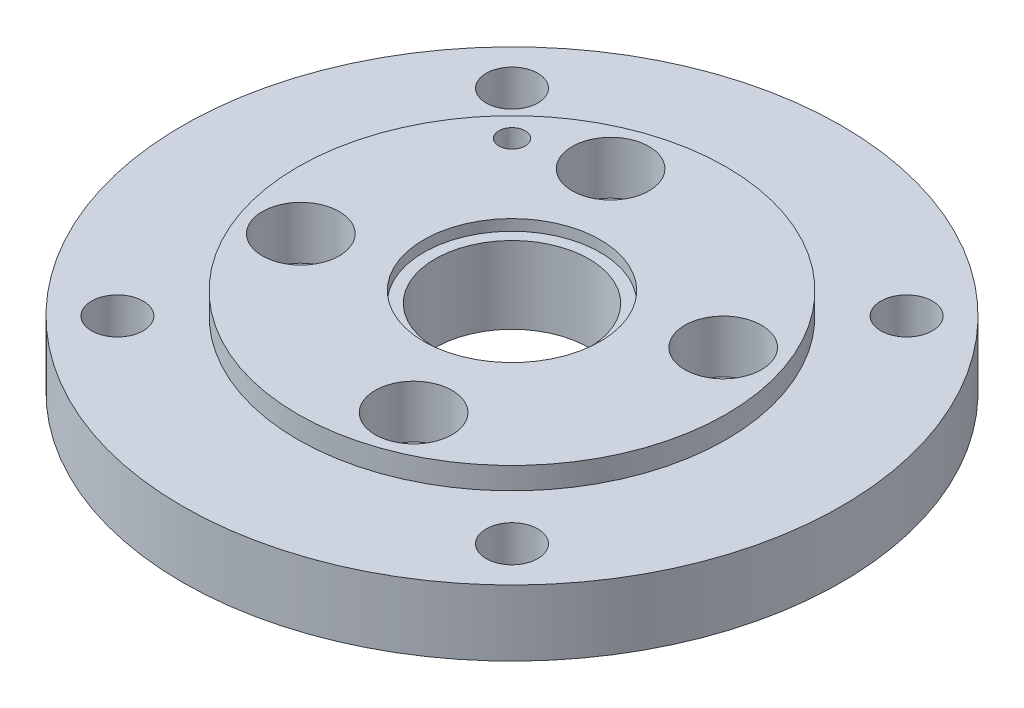
ISO-10303-21;
HEADER;
FILE_DESCRIPTION(('STEP AP214'),'2;1');
FILE_NAME('part.step','',(''),(''),'','','');
FILE_SCHEMA(('AUTOMOTIVE_DESIGN { 1 0 10303 214 1 1 1 1 }'));
ENDSEC;
DATA;
#1=APPLICATION_CONTEXT('core data for automotive mechanical design processes');
#2=APPLICATION_PROTOCOL_DEFINITION('international standard','automotive_design',2000,#1);
#3=PRODUCT_CONTEXT('',#1,'mechanical');
#4=PRODUCT('Part','Part','',(#3));
#5=PRODUCT_RELATED_PRODUCT_CATEGORY('part','',(#4));
#6=PRODUCT_DEFINITION_FORMATION('','',#4);
#7=PRODUCT_DEFINITION_CONTEXT('part definition',#1,'design');
#8=PRODUCT_DEFINITION('design','',#6,#7);
#9=PRODUCT_DEFINITION_SHAPE('','',#8);
#10=(LENGTH_UNIT() NAMED_UNIT(*) SI_UNIT(.MILLI.,.METRE.));
#11=(NAMED_UNIT(*) PLANE_ANGLE_UNIT() SI_UNIT($,.RADIAN.));
#12=(NAMED_UNIT(*) SI_UNIT($,.STERADIAN.) SOLID_ANGLE_UNIT());
#13=UNCERTAINTY_MEASURE_WITH_UNIT(LENGTH_MEASURE(1.E-05),#10,'distance_accuracy_value','');
#14=(GEOMETRIC_REPRESENTATION_CONTEXT(3) GLOBAL_UNCERTAINTY_ASSIGNED_CONTEXT((#13)) GLOBAL_UNIT_ASSIGNED_CONTEXT((#10,
#11,#12)) REPRESENTATION_CONTEXT('',''));
#15=CARTESIAN_POINT('',(0.,0.,0.));
#16=DIRECTION('',(0.,0.,1.));
#17=DIRECTION('',(1.,0.,0.));
#18=AXIS2_PLACEMENT_3D('',#15,#16,#17);
#19=CARTESIAN_POINT('',(0.,0.,0.));
#20=DIRECTION('',(0.,1.,0.));
#21=DIRECTION('',(0.,0.,1.));
#22=AXIS2_PLACEMENT_3D('',#19,#20,#21);
#23=PLANE('',#22);
#24=CARTESIAN_POINT('',(-60.,0.,-60.));
#25=DIRECTION('',(0.,1.,0.));
#26=DIRECTION('',(0.,0.,1.));
#27=AXIS2_PLACEMENT_3D('',#24,#25,#26);
#28=CIRCLE('',#27,6.);
#29=CARTESIAN_POINT('',(-60.,0.,-54.));
#30=VERTEX_POINT('',#29);
#31=EDGE_CURVE('E417',#30,#30,#28,.T.);
#32=ORIENTED_EDGE('',*,*,#31,.F.);
#33=EDGE_LOOP('',(#32));
#34=FACE_BOUND('',#33,.T.);
#35=CARTESIAN_POINT('',(-70.476946558943,0.,25.6515107494257));
#36=DIRECTION('',(0.,1.,0.));
#37=DIRECTION('',(0.,0.,1.));
#38=AXIS2_PLACEMENT_3D('',#35,#36,#37);
#39=CIRCLE('',#38,17.5);
#40=CARTESIAN_POINT('',(-70.476946558943,0.,43.1515107494257));
#41=VERTEX_POINT('',#40);
#42=EDGE_CURVE('E74',#41,#41,#39,.F.);
#43=ORIENTED_EDGE('',*,*,#42,.T.);
#44=EDGE_LOOP('',(#43));
#45=FACE_BOUND('',#44,.T.);
#46=CARTESIAN_POINT('',(25.686255304837,0.,70.4642908742771));
#47=DIRECTION('',(0.,1.,0.));
#48=DIRECTION('',(0.,0.,1.));
#49=AXIS2_PLACEMENT_3D('',#46,#47,#48);
#50=CIRCLE('',#49,17.5);
#51=CARTESIAN_POINT('',(25.686255304837,0.,87.9642908742771));
#52=VERTEX_POINT('',#51);
#53=EDGE_CURVE('E64',#52,#52,#50,.F.);
#54=ORIENTED_EDGE('',*,*,#53,.T.);
#55=EDGE_LOOP('',(#54));
#56=FACE_BOUND('',#55,.T.);
#57=CARTESIAN_POINT('',(0.,0.,0.));
#58=DIRECTION('',(0.,1.,0.));
#59=DIRECTION('',(0.,0.,1.));
#60=AXIS2_PLACEMENT_3D('',#57,#58,#59);
#61=CIRCLE('',#60,40.15);
#62=CARTESIAN_POINT('',(0.,0.,40.15));
#63=VERTEX_POINT('',#62);
#64=EDGE_CURVE('E113',#63,#63,#61,.T.);
#65=ORIENTED_EDGE('',*,*,#64,.F.);
#66=EDGE_LOOP('',(#65));
#67=FACE_BOUND('',#66,.T.);
#68=CARTESIAN_POINT('',(0.,0.,0.));
#69=DIRECTION('',(0.,1.,0.));
#70=DIRECTION('',(0.,0.,1.));
#71=AXIS2_PLACEMENT_3D('',#68,#69,#70);
#72=CIRCLE('',#71,97.5);
#73=CARTESIAN_POINT('',(0.,0.,97.5));
#74=VERTEX_POINT('',#73);
#75=EDGE_CURVE('E101',#74,#74,#72,.T.);
#76=ORIENTED_EDGE('',*,*,#75,.T.);
#77=EDGE_LOOP('',(#76));
#78=FACE_BOUND('',#77,.T.);
#79=CARTESIAN_POINT('',(70.4769465589431,0.,-25.6515107494252));
#80=DIRECTION('',(0.,1.,0.));
#81=DIRECTION('',(0.,0.,1.));
#82=AXIS2_PLACEMENT_3D('',#79,#80,#81);
#83=CIRCLE('',#82,17.5);
#84=CARTESIAN_POINT('',(70.4769465589431,0.,-8.15151074942521));
#85=VERTEX_POINT('',#84);
#86=EDGE_CURVE('E128',#85,#85,#83,.T.);
#87=ORIENTED_EDGE('',*,*,#86,.F.);
#88=EDGE_LOOP('',(#87));
#89=FACE_BOUND('',#88,.T.);
#90=CARTESIAN_POINT('',(-25.616759958528,0.,-70.4895851117536));
#91=DIRECTION('',(0.,1.,0.));
#92=DIRECTION('',(0.,0.,1.));
#93=AXIS2_PLACEMENT_3D('',#90,#91,#92);
#94=CIRCLE('',#93,17.5);
#95=CARTESIAN_POINT('',(-25.616759958528,0.,-52.9895851117536));
#96=VERTEX_POINT('',#95);
#97=EDGE_CURVE('E131',#96,#96,#94,.T.);
#98=ORIENTED_EDGE('',*,*,#97,.F.);
#99=EDGE_LOOP('',(#98));
#100=FACE_BOUND('',#99,.T.);
#101=ADVANCED_FACE('F40',(#34,#45,#56,#67,#78,#89,#100),#23,.T.);
#102=CARTESIAN_POINT('',(0.,-40.,0.));
#103=DIRECTION('',(0.,1.,0.));
#104=DIRECTION('',(0.,0.,1.));
#105=AXIS2_PLACEMENT_3D('',#102,#103,#104);
#106=CYLINDRICAL_SURFACE('',#105,150.);
#107=CARTESIAN_POINT('',(0.,-40.,0.));
#108=DIRECTION('',(0.,1.,0.));
#109=DIRECTION('',(0.,0.,1.));
#110=AXIS2_PLACEMENT_3D('',#107,#108,#109);
#111=CIRCLE('',#110,150.);
#112=CARTESIAN_POINT('',(0.,-40.,150.));
#113=VERTEX_POINT('',#112);
#114=EDGE_CURVE('E10',#113,#113,#111,.T.);
#115=ORIENTED_EDGE('',*,*,#114,.T.);
#116=EDGE_LOOP('',(#115));
#117=FACE_BOUND('',#116,.T.);
#118=CARTESIAN_POINT('',(0.,-10.,0.));
#119=DIRECTION('',(0.,1.,0.));
#120=DIRECTION('',(0.,0.,1.));
#121=AXIS2_PLACEMENT_3D('',#118,#119,#120);
#122=CIRCLE('',#121,150.);
#123=CARTESIAN_POINT('',(0.,-10.,150.));
#124=VERTEX_POINT('',#123);
#125=EDGE_CURVE('E110',#124,#124,#122,.T.);
#126=ORIENTED_EDGE('',*,*,#125,.F.);
#127=EDGE_LOOP('',(#126));
#128=FACE_BOUND('',#127,.T.);
#129=ADVANCED_FACE('F39',(#117,#128),#106,.T.);
#130=CARTESIAN_POINT('',(0.,-40.,0.));
#131=DIRECTION('',(0.,1.,0.));
#132=DIRECTION('',(0.,0.,1.));
#133=AXIS2_PLACEMENT_3D('',#130,#131,#132);
#134=CYLINDRICAL_SURFACE('',#133,35.);
#135=CARTESIAN_POINT('',(0.,-40.,0.));
#136=DIRECTION('',(0.,1.,0.));
#137=DIRECTION('',(0.,0.,1.));
#138=AXIS2_PLACEMENT_3D('',#135,#136,#137);
#139=CIRCLE('',#138,35.);
#140=CARTESIAN_POINT('',(0.,-40.,35.));
#141=VERTEX_POINT('',#140);
#142=EDGE_CURVE('E44',#141,#141,#139,.T.);
#143=ORIENTED_EDGE('',*,*,#142,.F.);
#144=EDGE_LOOP('',(#143));
#145=FACE_BOUND('',#144,.T.);
#146=CARTESIAN_POINT('',(0.,-5.,0.));
#147=DIRECTION('',(0.,1.,0.));
#148=DIRECTION('',(0.,0.,1.));
#149=AXIS2_PLACEMENT_3D('',#146,#147,#148);
#150=CIRCLE('',#149,35.);
#151=CARTESIAN_POINT('',(0.,-5.,35.));
#152=VERTEX_POINT('',#151);
#153=EDGE_CURVE('E115',#152,#152,#150,.T.);
#154=ORIENTED_EDGE('',*,*,#153,.T.);
#155=EDGE_LOOP('',(#154));
#156=FACE_BOUND('',#155,.T.);
#157=ADVANCED_FACE('F204',(#145,#156),#134,.F.);
#158=CARTESIAN_POINT('',(0.,-40.,0.));
#159=DIRECTION('',(0.,1.,0.));
#160=DIRECTION('',(0.,0.,1.));
#161=AXIS2_PLACEMENT_3D('',#158,#159,#160);
#162=PLANE('',#161);
#163=CARTESIAN_POINT('',(-60.,-40.,-60.));
#164=DIRECTION('',(0.,1.,0.));
#165=DIRECTION('',(0.,0.,1.));
#166=AXIS2_PLACEMENT_3D('',#163,#164,#165);
#167=CIRCLE('',#166,6.);
#168=CARTESIAN_POINT('',(-60.,-40.,-54.));
#169=VERTEX_POINT('',#168);
#170=EDGE_CURVE('E216',#169,#169,#167,.T.);
#171=ORIENTED_EDGE('',*,*,#170,.T.);
#172=EDGE_LOOP('',(#171));
#173=FACE_BOUND('',#172,.T.);
#174=CARTESIAN_POINT('',(70.4769465589431,-40.,-25.6515107494252));
#175=DIRECTION('',(0.,1.,0.));
#176=DIRECTION('',(0.,0.,1.));
#177=AXIS2_PLACEMENT_3D('',#174,#175,#176);
#178=CIRCLE('',#177,11.5);
#179=CARTESIAN_POINT('',(70.4769465589431,-40.,-14.1515107494252));
#180=VERTEX_POINT('',#179);
#181=EDGE_CURVE('E59',#180,#180,#178,.T.);
#182=ORIENTED_EDGE('',*,*,#181,.T.);
#183=EDGE_LOOP('',(#182));
#184=FACE_BOUND('',#183,.T.);
#185=CARTESIAN_POINT('',(-70.4074512126341,-40.,25.6262165119488));
#186=DIRECTION('',(0.,1.,0.));
#187=DIRECTION('',(0.,0.,-1.));
#188=AXIS2_PLACEMENT_3D('',#185,#186,#187);
#189=CIRCLE('',#188,11.5);
#190=CARTESIAN_POINT('',(-70.4074512126341,-40.,14.1262165119488));
#191=VERTEX_POINT('',#190);
#192=EDGE_CURVE('E224',#191,#191,#189,.T.);
#193=ORIENTED_EDGE('',*,*,#192,.T.);
#194=EDGE_LOOP('',(#193));
#195=FACE_BOUND('',#194,.T.);
#196=CARTESIAN_POINT('',(-25.616759958528,-40.,-70.4895851117536));
#197=DIRECTION('',(0.,1.,0.));
#198=DIRECTION('',(0.,0.,1.));
#199=AXIS2_PLACEMENT_3D('',#196,#197,#198);
#200=CIRCLE('',#199,11.5);
#201=CARTESIAN_POINT('',(-25.616759958528,-40.,-58.9895851117536));
#202=VERTEX_POINT('',#201);
#203=EDGE_CURVE('E230',#202,#202,#200,.T.);
#204=ORIENTED_EDGE('',*,*,#203,.T.);
#205=EDGE_LOOP('',(#204));
#206=FACE_BOUND('',#205,.T.);
#207=CARTESIAN_POINT('',(25.686255304837,-40.,70.4642908742771));
#208=DIRECTION('',(0.,1.,0.));
#209=DIRECTION('',(0.,0.,-1.));
#210=AXIS2_PLACEMENT_3D('',#207,#208,#209);
#211=CIRCLE('',#210,11.5000000000005);
#212=CARTESIAN_POINT('',(25.686255304837,-40.,58.9642908742766));
#213=VERTEX_POINT('',#212);
#214=EDGE_CURVE('E231',#213,#213,#211,.T.);
#215=ORIENTED_EDGE('',*,*,#214,.T.);
#216=EDGE_LOOP('',(#215));
#217=FACE_BOUND('',#216,.T.);
#218=CARTESIAN_POINT('',(89.8025612106914,-40.,89.8025612106917));
#219=DIRECTION('',(0.,1.,0.));
#220=DIRECTION('',(0.,0.,-1.));
#221=AXIS2_PLACEMENT_3D('',#218,#219,#220);
#222=CIRCLE('',#221,11.75);
#223=CARTESIAN_POINT('',(89.8025612106914,-40.,78.0525612106917));
#224=VERTEX_POINT('',#223);
#225=EDGE_CURVE('E93',#224,#224,#222,.T.);
#226=ORIENTED_EDGE('',*,*,#225,.T.);
#227=EDGE_LOOP('',(#226));
#228=FACE_BOUND('',#227,.T.);
#229=CARTESIAN_POINT('',(-89.8025612106914,-40.,89.8025612106917));
#230=DIRECTION('',(0.,1.,0.));
#231=DIRECTION('',(0.,0.,1.));
#232=AXIS2_PLACEMENT_3D('',#229,#230,#231);
#233=CIRCLE('',#232,11.75);
#234=CARTESIAN_POINT('',(-89.8025612106914,-40.,101.552561210692));
#235=VERTEX_POINT('',#234);
#236=EDGE_CURVE('E85',#235,#235,#233,.T.);
#237=ORIENTED_EDGE('',*,*,#236,.T.);
#238=EDGE_LOOP('',(#237));
#239=FACE_BOUND('',#238,.T.);
#240=CARTESIAN_POINT('',(-89.8025612106914,-40.,-89.8025612106917));
#241=DIRECTION('',(0.,1.,0.));
#242=DIRECTION('',(0.,0.,-1.));
#243=AXIS2_PLACEMENT_3D('',#240,#241,#242);
#244=CIRCLE('',#243,11.75);
#245=CARTESIAN_POINT('',(-89.8025612106914,-40.,-101.552561210692));
#246=VERTEX_POINT('',#245);
#247=EDGE_CURVE('E76',#246,#246,#244,.T.);
#248=ORIENTED_EDGE('',*,*,#247,.T.);
#249=EDGE_LOOP('',(#248));
#250=FACE_BOUND('',#249,.T.);
#251=CARTESIAN_POINT('',(89.8025612106914,-40.,-89.8025612106917));
#252=DIRECTION('',(0.,1.,0.));
#253=DIRECTION('',(0.,0.,1.));
#254=AXIS2_PLACEMENT_3D('',#251,#252,#253);
#255=CIRCLE('',#254,11.75);
#256=CARTESIAN_POINT('',(89.8025612106914,-40.,-78.0525612106917));
#257=VERTEX_POINT('',#256);
#258=EDGE_CURVE('E98',#257,#257,#255,.T.);
#259=ORIENTED_EDGE('',*,*,#258,.T.);
#260=EDGE_LOOP('',(#259));
#261=FACE_BOUND('',#260,.T.);
#262=ORIENTED_EDGE('',*,*,#142,.T.);
#263=EDGE_LOOP('',(#262));
#264=FACE_BOUND('',#263,.T.);
#265=ORIENTED_EDGE('',*,*,#114,.F.);
#266=EDGE_LOOP('',(#265));
#267=FACE_BOUND('',#266,.T.);
#268=ADVANCED_FACE('F205',(#173,#184,#195,#206,#217,#228,#239,#250,#261,#264,#267),#162,.F.);
#269=CARTESIAN_POINT('',(0.,-5.,0.));
#270=DIRECTION('',(0.,1.,0.));
#271=DIRECTION('',(0.,0.,1.));
#272=AXIS2_PLACEMENT_3D('',#269,#270,#271);
#273=CYLINDRICAL_SURFACE('',#272,40.15);
#274=CARTESIAN_POINT('',(0.,-5.,0.));
#275=DIRECTION('',(0.,1.,0.));
#276=DIRECTION('',(0.,0.,1.));
#277=AXIS2_PLACEMENT_3D('',#274,#275,#276);
#278=CIRCLE('',#277,40.15);
#279=CARTESIAN_POINT('',(0.,-5.,40.15));
#280=VERTEX_POINT('',#279);
#281=EDGE_CURVE('E49',#280,#280,#278,.T.);
#282=ORIENTED_EDGE('',*,*,#281,.F.);
#283=EDGE_LOOP('',(#282));
#284=FACE_BOUND('',#283,.T.);
#285=ORIENTED_EDGE('',*,*,#64,.T.);
#286=EDGE_LOOP('',(#285));
#287=FACE_BOUND('',#286,.T.);
#288=ADVANCED_FACE('F119',(#284,#287),#273,.F.);
#289=CARTESIAN_POINT('',(0.,-5.,0.));
#290=DIRECTION('',(0.,1.,0.));
#291=DIRECTION('',(0.,0.,1.));
#292=AXIS2_PLACEMENT_3D('',#289,#290,#291);
#293=PLANE('',#292);
#294=ORIENTED_EDGE('',*,*,#153,.F.);
#295=EDGE_LOOP('',(#294));
#296=FACE_BOUND('',#295,.T.);
#297=ORIENTED_EDGE('',*,*,#281,.T.);
#298=EDGE_LOOP('',(#297));
#299=FACE_BOUND('',#298,.T.);
#300=ADVANCED_FACE('F195',(#296,#299),#293,.T.);
#301=CARTESIAN_POINT('',(0.,-10.,0.));
#302=DIRECTION('',(0.,1.,0.));
#303=DIRECTION('',(0.,0.,1.));
#304=AXIS2_PLACEMENT_3D('',#301,#302,#303);
#305=PLANE('',#304);
#306=CARTESIAN_POINT('',(89.8025612106914,-10.,89.8025612106917));
#307=DIRECTION('',(0.,1.,0.));
#308=DIRECTION('',(0.,0.,-1.));
#309=AXIS2_PLACEMENT_3D('',#306,#307,#308);
#310=CIRCLE('',#309,11.75);
#311=CARTESIAN_POINT('',(89.8025612106914,-10.,78.0525612106917));
#312=VERTEX_POINT('',#311);
#313=EDGE_CURVE('E94',#312,#312,#310,.T.);
#314=ORIENTED_EDGE('',*,*,#313,.F.);
#315=EDGE_LOOP('',(#314));
#316=FACE_BOUND('',#315,.T.);
#317=CARTESIAN_POINT('',(-89.8025612106914,-10.,89.8025612106917));
#318=DIRECTION('',(0.,1.,0.));
#319=DIRECTION('',(0.,0.,1.));
#320=AXIS2_PLACEMENT_3D('',#317,#318,#319);
#321=CIRCLE('',#320,11.75);
#322=CARTESIAN_POINT('',(-89.8025612106914,-10.,101.552561210692));
#323=VERTEX_POINT('',#322);
#324=EDGE_CURVE('E86',#323,#323,#321,.T.);
#325=ORIENTED_EDGE('',*,*,#324,.F.);
#326=EDGE_LOOP('',(#325));
#327=FACE_BOUND('',#326,.T.);
#328=CARTESIAN_POINT('',(-89.8025612106914,-10.,-89.8025612106917));
#329=DIRECTION('',(0.,1.,0.));
#330=DIRECTION('',(0.,0.,-1.));
#331=AXIS2_PLACEMENT_3D('',#328,#329,#330);
#332=CIRCLE('',#331,11.75);
#333=CARTESIAN_POINT('',(-89.8025612106914,-10.,-101.552561210692));
#334=VERTEX_POINT('',#333);
#335=EDGE_CURVE('E82',#334,#334,#332,.T.);
#336=ORIENTED_EDGE('',*,*,#335,.F.);
#337=EDGE_LOOP('',(#336));
#338=FACE_BOUND('',#337,.T.);
#339=CARTESIAN_POINT('',(89.8025612106914,-10.,-89.8025612106917));
#340=DIRECTION('',(0.,1.,0.));
#341=DIRECTION('',(0.,0.,1.));
#342=AXIS2_PLACEMENT_3D('',#339,#340,#341);
#343=CIRCLE('',#342,11.75);
#344=CARTESIAN_POINT('',(89.8025612106914,-10.,-78.0525612106917));
#345=VERTEX_POINT('',#344);
#346=EDGE_CURVE('E81',#345,#345,#343,.T.);
#347=ORIENTED_EDGE('',*,*,#346,.F.);
#348=EDGE_LOOP('',(#347));
#349=FACE_BOUND('',#348,.T.);
#350=CARTESIAN_POINT('',(0.,-10.,0.));
#351=DIRECTION('',(0.,1.,0.));
#352=DIRECTION('',(0.,0.,1.));
#353=AXIS2_PLACEMENT_3D('',#350,#351,#352);
#354=CIRCLE('',#353,97.5);
#355=CARTESIAN_POINT('',(0.,-10.,97.5));
#356=VERTEX_POINT('',#355);
#357=EDGE_CURVE('E102',#356,#356,#354,.T.);
#358=ORIENTED_EDGE('',*,*,#357,.F.);
#359=EDGE_LOOP('',(#358));
#360=FACE_BOUND('',#359,.T.);
#361=ORIENTED_EDGE('',*,*,#125,.T.);
#362=EDGE_LOOP('',(#361));
#363=FACE_BOUND('',#362,.T.);
#364=ADVANCED_FACE('F191',(#316,#327,#338,#349,#360,#363),#305,.T.);
#365=CARTESIAN_POINT('',(0.,-10.,0.));
#366=DIRECTION('',(0.,1.,0.));
#367=DIRECTION('',(0.,0.,1.));
#368=AXIS2_PLACEMENT_3D('',#365,#366,#367);
#369=CYLINDRICAL_SURFACE('',#368,97.5);
#370=ORIENTED_EDGE('',*,*,#357,.T.);
#371=EDGE_LOOP('',(#370));
#372=FACE_BOUND('',#371,.T.);
#373=ORIENTED_EDGE('',*,*,#75,.F.);
#374=EDGE_LOOP('',(#373));
#375=FACE_BOUND('',#374,.T.);
#376=ADVANCED_FACE('F190',(#372,#375),#369,.T.);
#377=CARTESIAN_POINT('',(89.8025612106914,-40.,-89.8025612106917));
#378=DIRECTION('',(0.,1.,0.));
#379=DIRECTION('',(0.,0.,1.));
#380=AXIS2_PLACEMENT_3D('',#377,#378,#379);
#381=CYLINDRICAL_SURFACE('',#380,11.75);
#382=ORIENTED_EDGE('',*,*,#258,.F.);
#383=EDGE_LOOP('',(#382));
#384=FACE_BOUND('',#383,.T.);
#385=ORIENTED_EDGE('',*,*,#346,.T.);
#386=EDGE_LOOP('',(#385));
#387=FACE_BOUND('',#386,.T.);
#388=ADVANCED_FACE('F177',(#384,#387),#381,.F.);
#389=CARTESIAN_POINT('',(-89.8025612106914,-40.,-89.8025612106917));
#390=DIRECTION('',(0.,1.,0.));
#391=DIRECTION('',(0.,0.,1.));
#392=AXIS2_PLACEMENT_3D('',#389,#390,#391);
#393=CYLINDRICAL_SURFACE('',#392,11.75);
#394=ORIENTED_EDGE('',*,*,#247,.F.);
#395=EDGE_LOOP('',(#394));
#396=FACE_BOUND('',#395,.T.);
#397=ORIENTED_EDGE('',*,*,#335,.T.);
#398=EDGE_LOOP('',(#397));
#399=FACE_BOUND('',#398,.T.);
#400=ADVANCED_FACE('F171',(#396,#399),#393,.F.);
#401=CARTESIAN_POINT('',(-89.8025612106914,-40.,89.8025612106917));
#402=DIRECTION('',(0.,1.,0.));
#403=DIRECTION('',(0.,0.,1.));
#404=AXIS2_PLACEMENT_3D('',#401,#402,#403);
#405=CYLINDRICAL_SURFACE('',#404,11.75);
#406=ORIENTED_EDGE('',*,*,#236,.F.);
#407=EDGE_LOOP('',(#406));
#408=FACE_BOUND('',#407,.T.);
#409=ORIENTED_EDGE('',*,*,#324,.T.);
#410=EDGE_LOOP('',(#409));
#411=FACE_BOUND('',#410,.T.);
#412=ADVANCED_FACE('F176',(#408,#411),#405,.F.);
#413=CARTESIAN_POINT('',(89.8025612106914,-40.,89.8025612106917));
#414=DIRECTION('',(0.,1.,0.));
#415=DIRECTION('',(0.,0.,1.));
#416=AXIS2_PLACEMENT_3D('',#413,#414,#415);
#417=CYLINDRICAL_SURFACE('',#416,11.75);
#418=ORIENTED_EDGE('',*,*,#225,.F.);
#419=EDGE_LOOP('',(#418));
#420=FACE_BOUND('',#419,.T.);
#421=ORIENTED_EDGE('',*,*,#313,.T.);
#422=EDGE_LOOP('',(#421));
#423=FACE_BOUND('',#422,.T.);
#424=ADVANCED_FACE('F173',(#420,#423),#417,.F.);
#425=CARTESIAN_POINT('',(25.686255304837,-24.,70.4642908742771));
#426=DIRECTION('',(0.,1.,0.));
#427=DIRECTION('',(0.,0.,1.));
#428=AXIS2_PLACEMENT_3D('',#425,#426,#427);
#429=CYLINDRICAL_SURFACE('',#428,17.5);
#430=CARTESIAN_POINT('',(25.686255304837,-24.,70.4642908742771));
#431=DIRECTION('',(0.,1.,0.));
#432=DIRECTION('',(0.,0.,1.));
#433=AXIS2_PLACEMENT_3D('',#430,#431,#432);
#434=CIRCLE('',#433,17.5);
#435=CARTESIAN_POINT('',(25.686255304837,-24.,87.9642908742771));
#436=VERTEX_POINT('',#435);
#437=EDGE_CURVE('E68',#436,#436,#434,.F.);
#438=ORIENTED_EDGE('',*,*,#437,.T.);
#439=EDGE_LOOP('',(#438));
#440=FACE_BOUND('',#439,.T.);
#441=ORIENTED_EDGE('',*,*,#53,.F.);
#442=EDGE_LOOP('',(#441));
#443=FACE_BOUND('',#442,.T.);
#444=ADVANCED_FACE('F164',(#440,#443),#429,.F.);
#445=CARTESIAN_POINT('',(0.,-24.,0.));
#446=DIRECTION('',(0.,1.,0.));
#447=DIRECTION('',(0.,0.,1.));
#448=AXIS2_PLACEMENT_3D('',#445,#446,#447);
#449=PLANE('',#448);
#450=CARTESIAN_POINT('',(25.686255304837,-24.,70.4642908742771));
#451=DIRECTION('',(0.,1.,0.));
#452=DIRECTION('',(0.,0.,1.));
#453=AXIS2_PLACEMENT_3D('',#450,#451,#452);
#454=CIRCLE('',#453,11.5000000000005);
#455=CARTESIAN_POINT('',(25.686255304837,-24.,81.9642908742776));
#456=VERTEX_POINT('',#455);
#457=EDGE_CURVE('E41',#456,#456,#454,.T.);
#458=ORIENTED_EDGE('',*,*,#457,.F.);
#459=EDGE_LOOP('',(#458));
#460=FACE_BOUND('',#459,.T.);
#461=ORIENTED_EDGE('',*,*,#437,.F.);
#462=EDGE_LOOP('',(#461));
#463=FACE_BOUND('',#462,.T.);
#464=ADVANCED_FACE('F153',(#460,#463),#449,.T.);
#465=CARTESIAN_POINT('',(-70.476946558943,-24.,25.6515107494257));
#466=DIRECTION('',(0.,1.,0.));
#467=DIRECTION('',(0.,0.,1.));
#468=AXIS2_PLACEMENT_3D('',#465,#466,#467);
#469=CYLINDRICAL_SURFACE('',#468,17.5);
#470=CARTESIAN_POINT('',(-70.476946558943,-24.,25.6515107494257));
#471=DIRECTION('',(0.,1.,0.));
#472=DIRECTION('',(0.,0.,1.));
#473=AXIS2_PLACEMENT_3D('',#470,#471,#472);
#474=CIRCLE('',#473,17.5);
#475=CARTESIAN_POINT('',(-70.476946558943,-24.,43.1515107494257));
#476=VERTEX_POINT('',#475);
#477=EDGE_CURVE('E145',#476,#476,#474,.F.);
#478=ORIENTED_EDGE('',*,*,#477,.T.);
#479=EDGE_LOOP('',(#478));
#480=FACE_BOUND('',#479,.T.);
#481=ORIENTED_EDGE('',*,*,#42,.F.);
#482=EDGE_LOOP('',(#481));
#483=FACE_BOUND('',#482,.T.);
#484=ADVANCED_FACE('F147',(#480,#483),#469,.F.);
#485=CARTESIAN_POINT('',(0.,-24.,0.));
#486=DIRECTION('',(0.,1.,0.));
#487=DIRECTION('',(0.,0.,1.));
#488=AXIS2_PLACEMENT_3D('',#485,#486,#487);
#489=PLANE('',#488);
#490=CARTESIAN_POINT('',(-70.4074512126341,-24.,25.6262165119488));
#491=DIRECTION('',(0.,1.,0.));
#492=DIRECTION('',(0.,0.,1.));
#493=AXIS2_PLACEMENT_3D('',#490,#491,#492);
#494=CIRCLE('',#493,11.5);
#495=CARTESIAN_POINT('',(-70.4074512126341,-24.,37.1262165119487));
#496=VERTEX_POINT('',#495);
#497=EDGE_CURVE('E58',#496,#496,#494,.T.);
#498=ORIENTED_EDGE('',*,*,#497,.F.);
#499=EDGE_LOOP('',(#498));
#500=FACE_BOUND('',#499,.T.);
#501=ORIENTED_EDGE('',*,*,#477,.F.);
#502=EDGE_LOOP('',(#501));
#503=FACE_BOUND('',#502,.T.);
#504=ADVANCED_FACE('F155',(#500,#503),#489,.T.);
#505=CARTESIAN_POINT('',(70.4769465589431,-24.,-25.6515107494252));
#506=DIRECTION('',(0.,1.,0.));
#507=DIRECTION('',(0.,0.,1.));
#508=AXIS2_PLACEMENT_3D('',#505,#506,#507);
#509=CYLINDRICAL_SURFACE('',#508,17.5);
#510=CARTESIAN_POINT('',(70.4769465589431,-24.,-25.6515107494252));
#511=DIRECTION('',(0.,1.,0.));
#512=DIRECTION('',(0.,0.,1.));
#513=AXIS2_PLACEMENT_3D('',#510,#511,#512);
#514=CIRCLE('',#513,17.5);
#515=CARTESIAN_POINT('',(70.4769465589431,-24.,-8.15151074942521));
#516=VERTEX_POINT('',#515);
#517=EDGE_CURVE('E134',#516,#516,#514,.T.);
#518=ORIENTED_EDGE('',*,*,#517,.F.);
#519=EDGE_LOOP('',(#518));
#520=FACE_BOUND('',#519,.T.);
#521=ORIENTED_EDGE('',*,*,#86,.T.);
#522=EDGE_LOOP('',(#521));
#523=FACE_BOUND('',#522,.T.);
#524=ADVANCED_FACE('F161',(#520,#523),#509,.F.);
#525=CARTESIAN_POINT('',(0.,-24.,0.));
#526=DIRECTION('',(0.,1.,0.));
#527=DIRECTION('',(0.,0.,1.));
#528=AXIS2_PLACEMENT_3D('',#525,#526,#527);
#529=PLANE('',#528);
#530=CARTESIAN_POINT('',(70.4769465589431,-24.,-25.6515107494252));
#531=DIRECTION('',(0.,1.,0.));
#532=DIRECTION('',(0.,0.,1.));
#533=AXIS2_PLACEMENT_3D('',#530,#531,#532);
#534=CIRCLE('',#533,11.5);
#535=CARTESIAN_POINT('',(70.4769465589431,-24.,-14.1515107494252));
#536=VERTEX_POINT('',#535);
#537=EDGE_CURVE('E60',#536,#536,#534,.T.);
#538=ORIENTED_EDGE('',*,*,#537,.F.);
#539=EDGE_LOOP('',(#538));
#540=FACE_BOUND('',#539,.T.);
#541=ORIENTED_EDGE('',*,*,#517,.T.);
#542=EDGE_LOOP('',(#541));
#543=FACE_BOUND('',#542,.T.);
#544=ADVANCED_FACE('F332',(#540,#543),#529,.T.);
#545=CARTESIAN_POINT('',(-25.616759958528,-24.,-70.4895851117536));
#546=DIRECTION('',(0.,1.,0.));
#547=DIRECTION('',(0.,0.,1.));
#548=AXIS2_PLACEMENT_3D('',#545,#546,#547);
#549=CYLINDRICAL_SURFACE('',#548,17.5);
#550=CARTESIAN_POINT('',(-25.616759958528,-24.,-70.4895851117536));
#551=DIRECTION('',(0.,1.,0.));
#552=DIRECTION('',(0.,0.,1.));
#553=AXIS2_PLACEMENT_3D('',#550,#551,#552);
#554=CIRCLE('',#553,17.5);
#555=CARTESIAN_POINT('',(-25.616759958528,-24.,-52.9895851117536));
#556=VERTEX_POINT('',#555);
#557=EDGE_CURVE('E100',#556,#556,#554,.T.);
#558=ORIENTED_EDGE('',*,*,#557,.F.);
#559=EDGE_LOOP('',(#558));
#560=FACE_BOUND('',#559,.T.);
#561=ORIENTED_EDGE('',*,*,#97,.T.);
#562=EDGE_LOOP('',(#561));
#563=FACE_BOUND('',#562,.T.);
#564=ADVANCED_FACE('F337',(#560,#563),#549,.F.);
#565=CARTESIAN_POINT('',(0.,-24.,0.));
#566=DIRECTION('',(0.,1.,0.));
#567=DIRECTION('',(0.,0.,1.));
#568=AXIS2_PLACEMENT_3D('',#565,#566,#567);
#569=PLANE('',#568);
#570=CARTESIAN_POINT('',(-25.616759958528,-24.,-70.4895851117536));
#571=DIRECTION('',(0.,1.,0.));
#572=DIRECTION('',(0.,0.,1.));
#573=AXIS2_PLACEMENT_3D('',#570,#571,#572);
#574=CIRCLE('',#573,11.5);
#575=CARTESIAN_POINT('',(-25.616759958528,-24.,-58.9895851117536));
#576=VERTEX_POINT('',#575);
#577=EDGE_CURVE('E53',#576,#576,#574,.T.);
#578=ORIENTED_EDGE('',*,*,#577,.F.);
#579=EDGE_LOOP('',(#578));
#580=FACE_BOUND('',#579,.T.);
#581=ORIENTED_EDGE('',*,*,#557,.T.);
#582=EDGE_LOOP('',(#581));
#583=FACE_BOUND('',#582,.T.);
#584=ADVANCED_FACE('F355',(#580,#583),#569,.T.);
#585=CARTESIAN_POINT('',(-25.616759958528,-40.,-70.4895851117536));
#586=DIRECTION('',(0.,1.,0.));
#587=DIRECTION('',(0.,0.,1.));
#588=AXIS2_PLACEMENT_3D('',#585,#586,#587);
#589=CYLINDRICAL_SURFACE('',#588,11.5);
#590=ORIENTED_EDGE('',*,*,#577,.T.);
#591=EDGE_LOOP('',(#590));
#592=FACE_BOUND('',#591,.T.);
#593=ORIENTED_EDGE('',*,*,#203,.F.);
#594=EDGE_LOOP('',(#593));
#595=FACE_BOUND('',#594,.T.);
#596=ADVANCED_FACE('F363',(#592,#595),#589,.F.);
#597=CARTESIAN_POINT('',(70.4769465589431,-40.,-25.6515107494252));
#598=DIRECTION('',(0.,1.,0.));
#599=DIRECTION('',(0.,0.,1.));
#600=AXIS2_PLACEMENT_3D('',#597,#598,#599);
#601=CYLINDRICAL_SURFACE('',#600,11.5);
#602=ORIENTED_EDGE('',*,*,#537,.T.);
#603=EDGE_LOOP('',(#602));
#604=FACE_BOUND('',#603,.T.);
#605=ORIENTED_EDGE('',*,*,#181,.F.);
#606=EDGE_LOOP('',(#605));
#607=FACE_BOUND('',#606,.T.);
#608=ADVANCED_FACE('F372',(#604,#607),#601,.F.);
#609=CARTESIAN_POINT('',(-70.4074512126341,-40.,25.6262165119488));
#610=DIRECTION('',(0.,1.,0.));
#611=DIRECTION('',(0.,0.,1.));
#612=AXIS2_PLACEMENT_3D('',#609,#610,#611);
#613=CYLINDRICAL_SURFACE('',#612,11.5);
#614=ORIENTED_EDGE('',*,*,#497,.T.);
#615=EDGE_LOOP('',(#614));
#616=FACE_BOUND('',#615,.T.);
#617=ORIENTED_EDGE('',*,*,#192,.F.);
#618=EDGE_LOOP('',(#617));
#619=FACE_BOUND('',#618,.T.);
#620=ADVANCED_FACE('F383',(#616,#619),#613,.F.);
#621=CARTESIAN_POINT('',(25.686255304837,-40.,70.4642908742771));
#622=DIRECTION('',(0.,1.,0.));
#623=DIRECTION('',(0.,0.,1.));
#624=AXIS2_PLACEMENT_3D('',#621,#622,#623);
#625=CYLINDRICAL_SURFACE('',#624,11.5000000000005);
#626=ORIENTED_EDGE('',*,*,#457,.T.);
#627=EDGE_LOOP('',(#626));
#628=FACE_BOUND('',#627,.T.);
#629=ORIENTED_EDGE('',*,*,#214,.F.);
#630=EDGE_LOOP('',(#629));
#631=FACE_BOUND('',#630,.T.);
#632=ADVANCED_FACE('F392',(#628,#631),#625,.F.);
#633=CARTESIAN_POINT('',(-60.,-40.,-60.));
#634=DIRECTION('',(0.,1.,0.));
#635=DIRECTION('',(0.,0.,1.));
#636=AXIS2_PLACEMENT_3D('',#633,#634,#635);
#637=CYLINDRICAL_SURFACE('',#636,6.);
#638=ORIENTED_EDGE('',*,*,#170,.F.);
#639=EDGE_LOOP('',(#638));
#640=FACE_BOUND('',#639,.T.);
#641=ORIENTED_EDGE('',*,*,#31,.T.);
#642=EDGE_LOOP('',(#641));
#643=FACE_BOUND('',#642,.T.);
#644=ADVANCED_FACE('F401',(#640,#643),#637,.F.);
#645=CLOSED_SHELL('',(#101,#129,#157,#268,#288,#300,#364,#376,#388,#400,#412,#424,#444,#464,
#484,#504,#524,#544,#564,#584,#596,#608,#620,#632,#644));
#646=MANIFOLD_SOLID_BREP('B2',#645);
#647=ADVANCED_BREP_SHAPE_REPRESENTATION('',(#18,#646),#14);
#648=SHAPE_DEFINITION_REPRESENTATION(#9,#647);
ENDSEC;
END-ISO-10303-21;
